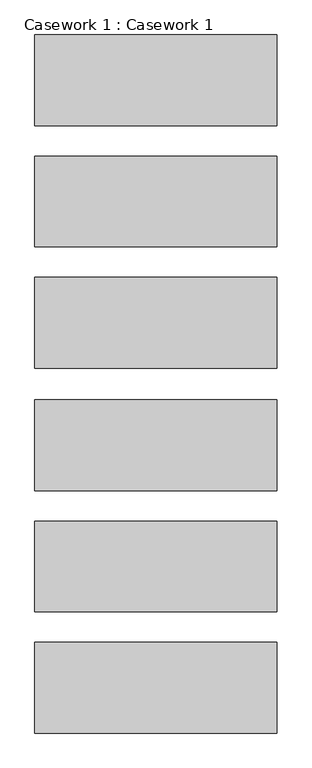
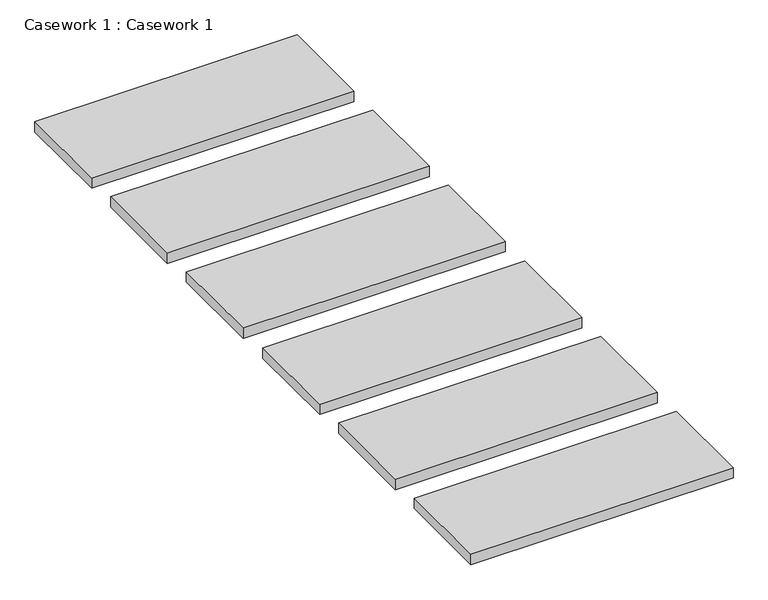
"""IFC4 building model written with IfcOpenShell, lengths in millimetres: furniture geometry, Casework 1 : Casework 1."""

from ifc_helpers import new_model, si_unit, frame, origin, place, context, project, spatial, polyline, outline, extrude, source, transform, mapped, element, save


def casework_1_casework_1_bf7433d0(model_context):
    return source(origin(), model_context, "Body", "SweptSolid", [
        extrude(outline(polyline([(-9767.6792561, -5626.7197682), (-8567.6792561, -5626.7197682), (-8567.6792561, -6076.7197682), (-9767.6792561, -6076.7197682), (-9767.6792561, -5626.7197682)])), frame((0.0, 0.0, 7275.0), z_axis=(0.0, 0.0, 1.0), x_axis=(1.0, 0.0, 0.0)), (0.0, 0.0, 1.0), 50.0),
        extrude(outline(polyline([(-9767.6792561, -5026.7197682), (-8567.6792561, -5026.7197682), (-8567.6792561, -5476.7197682), (-9767.6792561, -5476.7197682), (-9767.6792561, -5026.7197682)])), frame((0.0, 0.0, 7275.0), z_axis=(0.0, 0.0, 1.0), x_axis=(1.0, 0.0, 0.0)), (0.0, 0.0, 1.0), 50.0),
        extrude(outline(polyline([(-9767.6792561, -4426.7197682), (-8567.6792561, -4426.7197682), (-8567.6792561, -4876.7197682), (-9767.6792561, -4876.7197682), (-9767.6792561, -4426.7197682)])), frame((0.0, 0.0, 7275.0), z_axis=(0.0, 0.0, 1.0), x_axis=(1.0, 0.0, 0.0)), (0.0, 0.0, 1.0), 50.0),
        extrude(outline(polyline([(-9767.6792561, -3819.2197682), (-8567.6792561, -3819.2197682), (-8567.6792561, -4269.2197682), (-9767.6792561, -4269.2197682), (-9767.6792561, -3819.2197682)])), frame((0.0, 0.0, 7275.0), z_axis=(0.0, 0.0, 1.0), x_axis=(1.0, 0.0, 0.0)), (0.0, 0.0, 1.0), 50.0),
        extrude(outline(polyline([(-9767.6792561, -3219.2197682), (-8567.6792561, -3219.2197682), (-8567.6792561, -3669.2197682), (-9767.6792561, -3669.2197682), (-9767.6792561, -3219.2197682)])), frame((0.0, 0.0, 7275.0), z_axis=(0.0, 0.0, 1.0), x_axis=(1.0, 0.0, 0.0)), (0.0, 0.0, 1.0), 50.0),
        extrude(outline(polyline([(-9767.6792561, -2619.2197682), (-8567.6792561, -2619.2197682), (-8567.6792561, -3069.2197682), (-9767.6792561, -3069.2197682), (-9767.6792561, -2619.2197682)])), frame((0.0, 0.0, 7275.0), z_axis=(0.0, 0.0, 1.0), x_axis=(1.0, 0.0, 0.0)), (0.0, 0.0, 1.0), 50.0),
    ])


if __name__ == "__main__":
    model = new_model("IFC4")
    model_context = context("Model", 3, world=origin())
    ifc_project = project(units=[si_unit("LENGTHUNIT", "METRE", prefix="MILLI")], contexts=[model_context])
    site = spatial("IfcSite", under=ifc_project)
    building = spatial("IfcBuilding", under=site)
    placement = place(None, origin())
    casework_1_casework_1_shape = casework_1_casework_1_bf7433d0(model_context)
    element("IfcFurniture", 1, ObjectType="Casework 1 : Casework 1", at=placement, inside=building, context=model_context, shape_type="MappedRepresentation", body=[
        mapped(casework_1_casework_1_shape, transform((0.0, 0.0, 0.0), x_axis=(1.0, 0.0, 0.0), y_axis=(0.0, 1.0, 0.0), z_axis=(0.0, 0.0, 1.0))),
    ])
    save(model, "model.ifc")

# Revit data of these elements
# Element 1 (IfcFurniture, "Casework 1 : Casework 1")
#   Materials on its faces: "00-white plaster(1)"
# Materials
#   "00-white plaster(1)": class "Masonry", colour RGB 229 229 229, transparency 1, Description = "Common brick", Cost = 0
